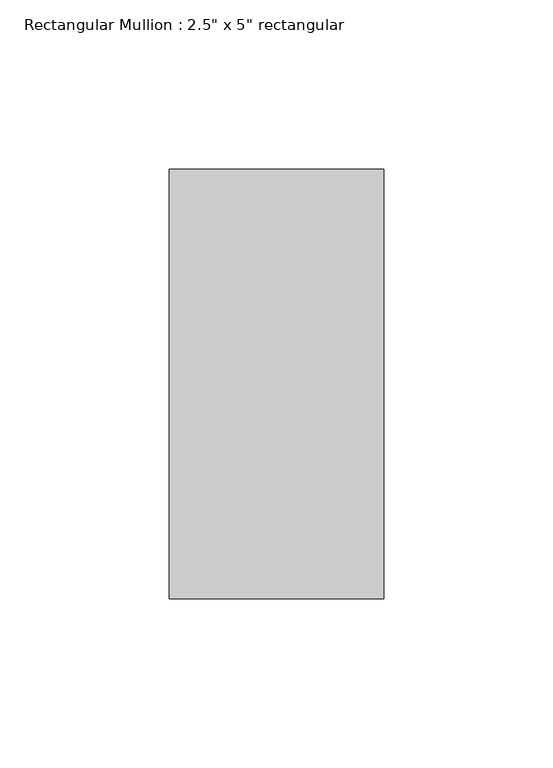
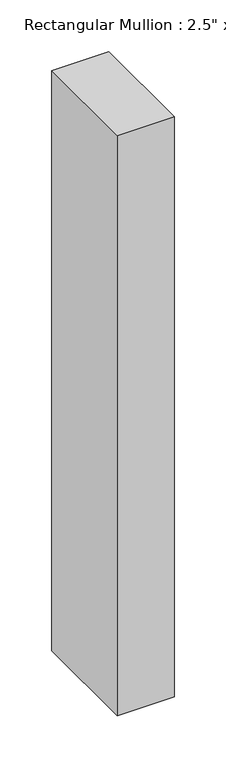
"""IFC4 building model written with IfcOpenShell, lengths in millimetres: member geometry."""

from ifc_helpers import new_model, si_unit, frame, origin, place, context, project, spatial, polyline, outline, extrude, source, transform, mapped, element, save


def member_2c92067c(model_context):
    return source(origin(), model_context, "Body", "SweptSolid", [
        extrude(outline(polyline([(31.75, 63.5), (31.75, -63.5), (-31.75, -63.5), (-31.75, 63.5), (31.75, 63.5)])), frame((0.0, 0.0, -685.4574877), z_axis=(0.0, 0.0, 1.0), x_axis=(1.0, 0.0, 0.0)), (0.0, 0.0, 1.0), 685.4574877),
    ])


if __name__ == "__main__":
    model = new_model("IFC4")
    model_context = context("Model", 3, world=origin())
    ifc_project = project(units=[si_unit("LENGTHUNIT", "METRE", prefix="MILLI")], contexts=[model_context])
    site = spatial("IfcSite", under=ifc_project)
    building = spatial("IfcBuilding", under=site)
    placement = place(None, origin())
    member_shape = member_2c92067c(model_context)
    element("IfcMember", 1, ObjectType="Rectangular Mullion : 2.5\" x 5\" rectangular", at=placement, inside=building, context=model_context, shape_type="MappedRepresentation", body=[
        mapped(member_shape, transform((0.0, 0.0, 0.0), x_axis=(1.0, 0.0, 0.0), y_axis=(0.0, 1.0, 0.0), z_axis=(0.0, 0.0, 1.0))),
    ])
    save(model, "model.ifc")

# Revit data of these elements
# Type "Rectangular Mullion : 2.5\" x 5\" rectangular"
#   built-in parameter 1007304 = 0.416667 (stored number, unit not read)
#   built-in parameter 1007301 = 0.104167 (stored number, unit not read)
#   built-in parameter 1007300 = 0.104167 (stored number, unit not read)
# Element 1 (IfcMember, "Rectangular Mullion : 2.5\" x 5\" rectangular")
#   Materials on its faces: "Aluminum"
# Materials
#   "Aluminum": class "Metal", colour RGB 247 247 247, transparency 0, Description = "Aluminum 6061", Cost = 0
